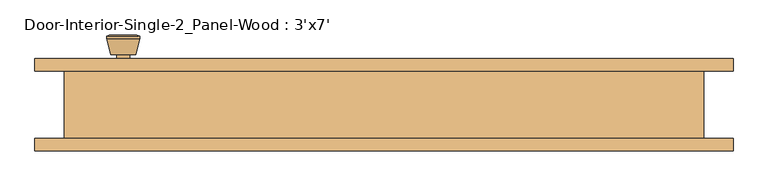
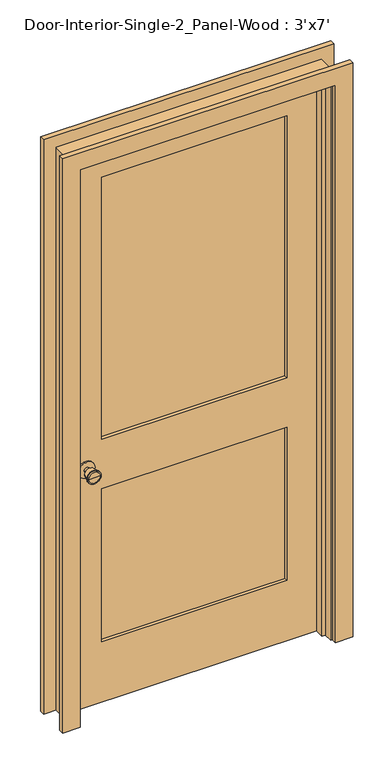
"""IFC4 building model written with IfcOpenShell, lengths in millimetres: door geometry, Door-Interior-Single-2_Panel-Wood : 3'x7'."""

from ifc_helpers import new_model, si_unit, point, frame, frame_2d, origin, place, context, project, spatial, polyline, circle_curve, trimmed, segment, composite_curve, outline, extrude, faceted_brep, source, transform, mapped, element, save
from ifc_brep_helpers import plane_surface, cylinder_surface, revolved_surface, advanced_brep


def door_interior_single_2_panel_wood_3_x7_894b38f8(model_context):
    return source(origin(), model_context, "Body", "SolidModel", [
        advanced_brep(
        [(-393.7, 6.7, 914.4), (-383.7, 6.7, 914.4), (-403.7, 6.7, 914.4), (-373.2241324, -42.3, 914.4), (-393.7, -42.3, 914.4), (-414.1758676, -42.3, 914.4), (-368.7, -40.4721319, 914.4), (-418.7, -40.4721319, 914.4), (-368.7, -37.0084537, 914.4), (-418.7, -37.0084537, 914.4), (-375.063764, -12.3, 914.4), (-412.336236, -12.3, 914.4), (-383.7, -12.3, 914.4), (-403.7, -12.3, 914.4)],
        [
            (0, 1),
            (1, 2, circle_curve(frame((-393.7, 6.7, 914.4), z_axis=(0.0, 1.0, 0.0), x_axis=(-1.0, 0.0, 0.0)), 10.0)),
            (2, 0),
            (2, 1, circle_curve(frame((-393.7, 6.7, 914.4), z_axis=(0.0, 1.0, 0.0), x_axis=(-1.0, 0.0, 0.0)), 10.0)),
            (3, 4),
            (4, 5),
            (5, 3, circle_curve(frame((-393.7, -42.3, 914.4), z_axis=(0.0, -1.0, 0.0), x_axis=(-1.0, 0.0, 0.0)), 20.4758676)),
            (3, 5, circle_curve(frame((-393.7, -42.3, 914.4), z_axis=(0.0, -1.0, 0.0), x_axis=(-1.0, 0.0, 0.0)), 20.4758676)),
            (6, 3),
            (5, 7),
            (7, 6, circle_curve(frame((-393.7, -40.4721319, 914.4), z_axis=(0.0, -1.0, 0.0), x_axis=(-1.0, 0.0, 0.0)), 25.0)),
            (6, 7, circle_curve(frame((-393.7, -40.4721319, 914.4), z_axis=(0.0, -1.0, 0.0), x_axis=(-1.0, 0.0, 0.0)), 25.0)),
            (8, 6),
            (7, 9),
            (9, 8, circle_curve(frame((-393.7, -37.0084537, 914.4), z_axis=(0.0, -1.0, 0.0), x_axis=(-1.0, 0.0, 0.0)), 25.0)),
            (8, 9, circle_curve(frame((-393.7, -37.0084537, 914.4), z_axis=(0.0, -1.0, 0.0), x_axis=(-1.0, 0.0, 0.0)), 25.0)),
            (10, 8),
            (9, 11),
            (11, 10, circle_curve(frame((-393.7, -12.3, 914.4), z_axis=(0.0, -1.0, 0.0), x_axis=(-1.0, 0.0, 0.0)), 18.636236)),
            (10, 11, circle_curve(frame((-393.7, -12.3, 914.4), z_axis=(0.0, -1.0, 0.0), x_axis=(-1.0, 0.0, 0.0)), 18.636236)),
            (12, 10),
            (11, 13),
            (13, 12, circle_curve(frame((-393.7, -12.3, 914.4), z_axis=(0.0, -1.0, 0.0), x_axis=(-1.0, 0.0, 0.0)), 10.0)),
            (12, 13, circle_curve(frame((-393.7, -12.3, 914.4), z_axis=(0.0, -1.0, 0.0), x_axis=(-1.0, 0.0, 0.0)), 10.0)),
            (1, 12),
            (13, 2),
        ],
        [
            plane_surface(frame((-393.7, 6.7, 914.4), z_axis=(0.0, 1.0, 0.0), x_axis=(-1.0, 0.0, 0.0))),
            plane_surface(frame((-393.7, -42.3, 914.4), z_axis=(0.0, -1.0, 0.0), x_axis=(-1.0, 0.0, 0.0))),
            revolved_surface(polyline([(-414.1758676, -42.3, 914.4), (-418.7, -40.4721319, 914.4)]), (-393.7, 6.7, 914.4), (0.0, 1.0, 0.0)),
            cylinder_surface(frame((-393.7, 6.7, 914.4), z_axis=(0.0, 1.0, 0.0), x_axis=(-1.0, 0.0, 0.0)), 25.0),
            revolved_surface(polyline([(-418.7, -37.0084537, 914.4), (-412.336236, -12.3, 914.4)]), (-393.7, 6.7, 914.4), (0.0, 1.0, 0.0)),
            plane_surface(frame((-393.7, -12.3, 914.4), z_axis=(0.0, 1.0, 0.0), x_axis=(-1.0, 0.0, 0.0))),
            cylinder_surface(frame((-393.7, 6.7, 914.4), z_axis=(0.0, 1.0, 0.0), x_axis=(-1.0, 0.0, 0.0)), 10.0),
        ],
        [
            (0, [[1, 2, 3]]),
            (0, [[-3, 4, -1]]),
            (1, [[5, 6, 7]]),
            (1, [[-6, -5, 8]]),
            (2, [[9, -7, 10, 11]]),
            (2, [[-10, -8, -9, 12]]),
            (3, [[13, -11, 14, 15]]),
            (3, [[-14, -12, -13, 16]]),
            (4, [[17, -15, 18, 19]]),
            (4, [[-18, -16, -17, 20]]),
            (5, [[21, -19, 22, 23]]),
            (5, [[-22, -20, -21, 24]]),
            (6, [[25, -23, 26, -2]]),
            (6, [[-26, -24, -25, -4]]),
        ],
    ),
        extrude(outline(composite_curve([segment(trimmed(circle_curve(frame_2d((914.4, -393.7)), 30.0), [point((914.4, -423.7))], [point((914.4, -363.7))], False, "CARTESIAN"), True, "CONTINUOUS"), segment(trimmed(circle_curve(frame_2d((914.4, -393.7)), 30.0), [point((914.4, -363.7))], [point((914.4, -423.7))], False, "CARTESIAN"), True, "CONTINUOUS")], self_intersect=False)), frame((0.0, 6.7, 0.0), z_axis=(0.0, 1.0, 0.0), x_axis=(0.0, 0.0, 1.0)), (0.0, 0.0, 1.0), 6.0),
        advanced_brep(
        [(-393.7, 53.625, 914.4), (-403.7, 53.625, 914.4), (-383.7, 53.625, 914.4), (-373.2241324, 102.625, 914.4), (-414.1758676, 102.625, 914.4), (-393.7, 102.625, 914.4), (-368.7, 100.7971319, 914.4), (-418.7, 100.7971319, 914.4), (-368.7, 97.3334537, 914.4), (-418.7, 97.3334537, 914.4), (-375.063764, 72.625, 914.4), (-412.336236, 72.625, 914.4), (-383.7, 72.625, 914.4), (-403.7, 72.625, 914.4)],
        [
            (0, 1),
            (1, 2, circle_curve(frame((-393.7, 53.625, 914.4), z_axis=(0.0, -1.0, 0.0), x_axis=(-1.0, 0.0, 0.0)), 10.0)),
            (2, 0),
            (2, 1, circle_curve(frame((-393.7, 53.625, 914.4), z_axis=(0.0, -1.0, 0.0), x_axis=(-1.0, 0.0, 0.0)), 10.0)),
            (3, 4, circle_curve(frame((-393.7, 102.625, 914.4), z_axis=(0.0, 1.0, 0.0), x_axis=(-1.0, 0.0, 0.0)), 20.4758676)),
            (4, 5),
            (5, 3),
            (4, 3, circle_curve(frame((-393.7, 102.625, 914.4), z_axis=(0.0, 1.0, 0.0), x_axis=(-1.0, 0.0, 0.0)), 20.4758676)),
            (6, 7, circle_curve(frame((-393.7, 100.7971319, 914.4), z_axis=(0.0, 1.0, 0.0), x_axis=(-1.0, 0.0, 0.0)), 25.0)),
            (7, 4),
            (3, 6),
            (7, 6, circle_curve(frame((-393.7, 100.7971319, 914.4), z_axis=(0.0, 1.0, 0.0), x_axis=(-1.0, 0.0, 0.0)), 25.0)),
            (8, 9, circle_curve(frame((-393.7, 97.3334537, 914.4), z_axis=(0.0, 1.0, 0.0), x_axis=(-1.0, 0.0, 0.0)), 25.0)),
            (9, 7),
            (6, 8),
            (9, 8, circle_curve(frame((-393.7, 97.3334537, 914.4), z_axis=(0.0, 1.0, 0.0), x_axis=(-1.0, 0.0, 0.0)), 25.0)),
            (10, 11, circle_curve(frame((-393.7, 72.625, 914.4), z_axis=(0.0, 1.0, 0.0), x_axis=(-1.0, 0.0, 0.0)), 18.636236)),
            (11, 9),
            (8, 10),
            (11, 10, circle_curve(frame((-393.7, 72.625, 914.4), z_axis=(0.0, 1.0, 0.0), x_axis=(-1.0, 0.0, 0.0)), 18.636236)),
            (12, 13, circle_curve(frame((-393.7, 72.625, 914.4), z_axis=(0.0, 1.0, 0.0), x_axis=(-1.0, 0.0, 0.0)), 10.0)),
            (13, 11),
            (10, 12),
            (13, 12, circle_curve(frame((-393.7, 72.625, 914.4), z_axis=(0.0, 1.0, 0.0), x_axis=(-1.0, 0.0, 0.0)), 10.0)),
            (1, 13),
            (12, 2),
        ],
        [
            plane_surface(frame((-393.7, 53.625, 914.4), z_axis=(0.0, -1.0, 0.0), x_axis=(-1.0, 0.0, 0.0))),
            plane_surface(frame((-393.7, 102.625, 914.4), z_axis=(0.0, 1.0, 0.0), x_axis=(-1.0, 0.0, 0.0))),
            revolved_surface(polyline([(-414.1758676, 102.625, 914.4), (-418.7, 100.7971319, 914.4)]), (-393.7, 53.625, 914.4), (0.0, -1.0, 0.0)),
            cylinder_surface(frame((-393.7, 53.625, 914.4), z_axis=(0.0, -1.0, 0.0), x_axis=(-1.0, 0.0, 0.0)), 25.0),
            revolved_surface(polyline([(-418.7, 97.3334537, 914.4), (-412.336236, 72.625, 914.4)]), (-393.7, 53.625, 914.4), (0.0, -1.0, 0.0)),
            plane_surface(frame((-393.7, 72.625, 914.4), z_axis=(0.0, -1.0, 0.0), x_axis=(-1.0, 0.0, 0.0))),
            cylinder_surface(frame((-393.7, 53.625, 914.4), z_axis=(0.0, -1.0, 0.0), x_axis=(-1.0, 0.0, 0.0)), 10.0),
        ],
        [
            (0, [[1, 2, 3]]),
            (0, [[-3, 4, -1]]),
            (1, [[5, 6, 7]]),
            (1, [[8, -7, -6]]),
            (2, [[9, 10, -5, 11]]),
            (2, [[12, -11, -8, -10]]),
            (3, [[13, 14, -9, 15]]),
            (3, [[16, -15, -12, -14]]),
            (4, [[17, 18, -13, 19]]),
            (4, [[20, -19, -16, -18]]),
            (5, [[21, 22, -17, 23]]),
            (5, [[24, -23, -20, -22]]),
            (6, [[-2, 25, -21, 26]]),
            (6, [[-4, -26, -24, -25]]),
        ],
    ),
        extrude(outline(composite_curve([segment(trimmed(circle_curve(frame_2d((914.4, -393.7)), 30.0), [point((914.4, -423.7))], [point((914.4, -363.7))], False, "CARTESIAN"), True, "CONTINUOUS"), segment(trimmed(circle_curve(frame_2d((914.4, -393.7)), 30.0), [point((914.4, -363.7))], [point((914.4, -423.7))], False, "CARTESIAN"), True, "CONTINUOUS")], self_intersect=False)), frame((0.0, 47.625, 0.0), z_axis=(0.0, 1.0, 0.0), x_axis=(0.0, 0.0, 1.0)), (0.0, 0.0, 1.0), 6.0),
        faceted_brep([(482.6, 47.625, 0.0), (482.6, -53.975, 0.0), (457.2, -53.975, 0.0), (457.2, -22.225, 0.0), (444.5, -22.225, 0.0), (444.5, 12.7, 0.0), (457.2, 12.7, 0.0), (457.2, 47.625, 0.0), (482.6, 47.625, 2159.0), (482.6, -53.975, 2159.0), (-482.6, -53.975, 2159.0), (-482.6, -53.975, 0.0), (-457.2, -53.975, 0.0), (-457.2, -53.975, 2133.6), (457.2, -53.975, 2133.6), (457.2, -22.225, 2133.6), (-457.2, -22.225, 2133.6), (-457.2, -22.225, 0.0), (-444.5, -22.225, 0.0), (-444.5, -22.225, 2120.9), (444.5, -22.225, 2120.9), (444.5, 12.7, 2120.9), (-444.5, 12.7, 2120.9), (-444.5, 12.7, 0.0), (-457.2, 12.7, 0.0), (-457.2, 12.7, 2133.6), (457.2, 12.7, 2133.6), (457.2, 47.625, 2133.6), (-457.2, 47.625, 2133.6), (-457.2, 47.625, 0.0), (-482.6, 47.625, 0.0), (-482.6, 47.625, 2159.0)], [[[0, 1, 2, 3, 4, 5, 6, 7]], [[1, 0, 8, 9]], [[2, 1, 9, 10, 11, 12, 13, 14]], [[3, 2, 14, 15]], [[4, 3, 15, 16, 17, 18, 19, 20]], [[5, 4, 20, 21]], [[6, 5, 21, 22, 23, 24, 25, 26]], [[7, 6, 26, 27]], [[0, 7, 27, 28, 29, 30, 31, 8]], [[9, 8, 31, 10]], [[15, 14, 13, 16]], [[21, 20, 19, 22]], [[27, 26, 25, 28]], [[30, 29, 24, 23, 18, 17, 12, 11]], [[10, 31, 30, 11]], [[16, 13, 12, 17]], [[22, 19, 18, 23]], [[28, 25, 24, 29]]]),
        extrude(outline(polyline([(2133.6, -457.2), (0.0, -457.2), (0.0, 457.2), (2133.6, 457.2), (2133.6, -457.2)]), holes=[polyline([(2014.5375, -336.55), (2014.5375, 336.55), (1009.65, 336.55), (1009.65, -336.55), (2014.5375, -336.55)]), polyline([(819.15, -336.55), (819.15, 336.55), (231.775, 336.55), (231.775, -336.55), (819.15, -336.55)])]), frame((0.0, 12.7, 0.0), z_axis=(0.0, 1.0, 0.0), x_axis=(0.0, 0.0, 1.0)), (0.0, 0.0, 1.0), 34.925),
        extrude(outline(polyline([(336.55, 24.3416667), (-336.55, 24.3416667), (-336.55, 35.9833333), (336.55, 35.9833333), (336.55, 24.3416667)])), frame((0.0, 0.0, 1009.65), z_axis=(0.0, 0.0, 1.0), x_axis=(1.0, 0.0, 0.0)), (0.0, 0.0, 1.0), 1004.8875),
        extrude(outline(polyline([(336.55, 24.3416667), (-336.55, 24.3416667), (-336.55, 35.9833333), (336.55, 35.9833333), (336.55, 24.3416667)])), frame((0.0, 0.0, 231.775), z_axis=(0.0, 0.0, 1.0), x_axis=(1.0, 0.0, 0.0)), (0.0, 0.0, 1.0), 587.375),
        extrude(outline(polyline([(0.0, 463.55), (0.0, 527.05), (2203.45, 527.05), (2203.45, -527.05), (0.0, -527.05), (0.0, -463.55), (2139.95, -463.55), (2139.95, 463.55), (0.0, 463.55)])), frame((0.0, 47.625, 0.0), z_axis=(0.0, 1.0, 0.0), x_axis=(0.0, 0.0, 1.0)), (0.0, 0.0, 1.0), 19.05),
        extrude(outline(polyline([(0.0, 463.55), (0.0, 527.05), (2203.45, 527.05), (2203.45, -527.05), (0.0, -527.05), (0.0, -463.55), (2139.95, -463.55), (2139.95, 463.55), (0.0, 463.55)])), frame((0.0, -73.025, 0.0), z_axis=(0.0, 1.0, 0.0), x_axis=(0.0, 0.0, 1.0)), (0.0, 0.0, 1.0), 19.05),
    ])


if __name__ == "__main__":
    model = new_model("IFC4")
    model_context = context("Model", 3, world=origin())
    ifc_project = project(units=[si_unit("LENGTHUNIT", "METRE", prefix="MILLI")], contexts=[model_context])
    site = spatial("IfcSite", under=ifc_project)
    building = spatial("IfcBuilding", under=site)
    placement = place(None, origin())
    door_interior_single_2_panel_wood_3_x7_shape = door_interior_single_2_panel_wood_3_x7_894b38f8(model_context)
    element("IfcDoor", 1, ObjectType="Door-Interior-Single-2_Panel-Wood : 3'x7'", at=placement, inside=building, context=model_context, shape_type="MappedRepresentation", body=[
        mapped(door_interior_single_2_panel_wood_3_x7_shape, transform((0.0, 0.0, 0.0), x_axis=(1.0, 0.0, 0.0), y_axis=(0.0, 1.0, 0.0), z_axis=(0.0, 0.0, 1.0))),
    ])
    save(model, "model.ifc")

# Revit data of these elements
# Type "Door-Interior-Single-2_Panel-Wood : 3'x7'"
#   Type Mark = "9"
#   Assembly Code = "C1020300"
#   Analytic Construction = "Wooden"
#   Top Rail = 0' - 4 11/16"
#   Thickness = 0' - 1 3/8"
#   Thermal Resistance (R) = 2.5876 (h·ft²·°F)/BTU
#   Swing Angle [instance default] = 90.00°
#   Stiles = 0' - 4 3/4"
#   Rough Width = 3' - 2"
#   Rough Height = 7' - 1"
#   Lock Rail = 0' - 7 1/2"
#   Height = 7' - 0"
#   Width = 3' - 0"
#   Heat Transfer Coefficient (U) = 0.3865 BTU/(h·ft²·°F)
#   Bottom Rail = 0' - 9 1/8"
#   Trim Material = Cherry
#   Panel Material = Cherry
#   Frame Material = Cherry
#   Door Handle Material = Aluminum
#   Visual Light Transmittance = 0
#   Solar Heat Gain Coefficient = 0
#   Wall Closure = (empty or 0)
#   Function = (empty or 0)
# Element 1 (IfcDoor, "Door-Interior-Single-2_Panel-Wood : 3'x7'")
#   Materials on its faces: "Cherry", "Aluminum"
# Materials
#   "Cherry": class "Wood", colour RGB 226 177 128, transparency 0, Description = "Prunus Serotina", Cost = 0
#   "Aluminum": class "Metal", colour RGB 247 247 247, transparency 0, Description = "Aluminum 6061", Cost = 0
